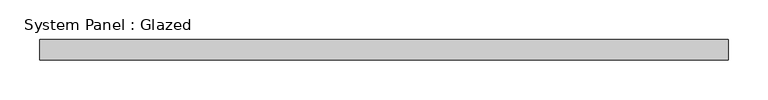
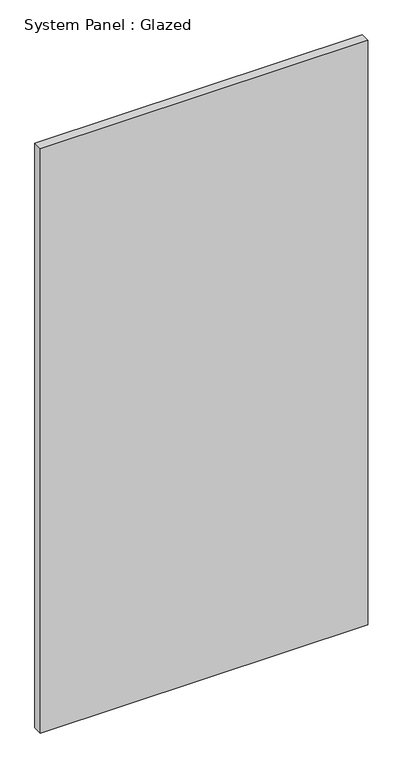
"""IFC4 building model written with IfcOpenShell, lengths in millimetres: plate geometry, System Panel : Glazed."""

from ifc_helpers import new_model, si_unit, origin, origin_with_axes, place, context, project, spatial, polyline, outline, extrude, source, transform, mapped, element, save


def system_panel_glazed_1c5a620b(model_context):
    return source(origin(), model_context, "Body", "SweptSolid", [
        extrude(outline(polyline([(431.8, 19.05), (-431.8, 19.05), (-431.8, 44.45), (431.8, 44.45), (431.8, 19.05)])), origin_with_axes(), (0.0, 0.0, 1.0), 1629.8052168),
    ])


if __name__ == "__main__":
    model = new_model("IFC4")
    model_context = context("Model", 3, world=origin())
    ifc_project = project(units=[si_unit("LENGTHUNIT", "METRE", prefix="MILLI")], contexts=[model_context])
    site = spatial("IfcSite", under=ifc_project)
    building = spatial("IfcBuilding", under=site)
    placement = place(None, origin())
    system_panel_glazed_shape = system_panel_glazed_1c5a620b(model_context)
    element("IfcPlate", 1, ObjectType="System Panel : Glazed", at=placement, inside=building, context=model_context, shape_type="MappedRepresentation", body=[
        mapped(system_panel_glazed_shape, transform((0.0, 0.0, 0.0), x_axis=(1.0, 0.0, 0.0), y_axis=(0.0, 1.0, 0.0), z_axis=(0.0, 0.0, 1.0))),
    ])
    save(model, "model.ifc")

# Revit data of these elements
# Type "System Panel : Glazed"
#   Construction Type Id = "GSP4R"
#   Analytic Construction = "1/8 in Pilkington single glazing"
#   Visual Light Transmittance = 0.9
#   Solar Heat Gain Coefficient = 0.86
#   Heat Transfer Coefficient (U) = 1.18115 BTU/(h·ft²·°F)
#   Define Thermal Properties by = 1
# Element 1 (IfcPlate, "System Panel : Glazed")
#   Materials on its faces: "Glass"
# Materials
#   "Glass": class "Glass", colour RGB 0 128 192, transparency 0.75, Description = "Soda Lime Glass", Cost = 0
